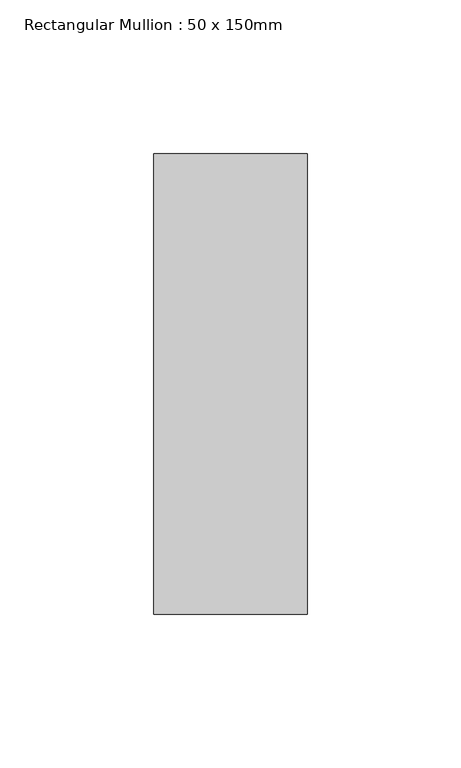
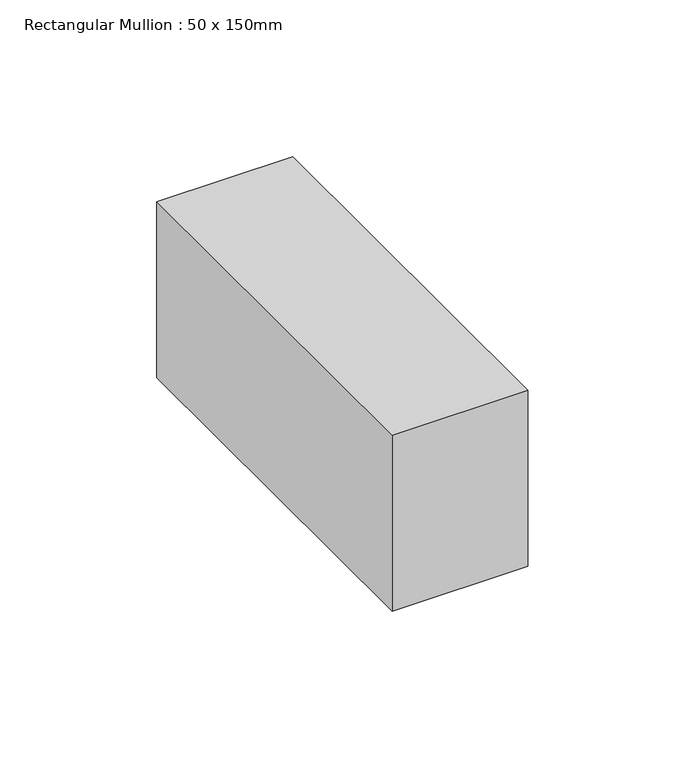
"""IFC4 building model written with IfcOpenShell, lengths in millimetres: member geometry, Rectangular Mullion : 50 x 150mm."""

from ifc_helpers import new_model, si_unit, frame, origin, place, context, project, spatial, polyline, outline, extrude, source, transform, mapped, element, save


def rectangular_mullion_50_x_150mm_e4b12c2e(model_context):
    return source(origin(), model_context, "Body", "SweptSolid", [
        extrude(outline(polyline([(0.0, 75.0), (0.0, -75.0), (-50.0, -75.0), (-50.0, 75.0), (0.0, 75.0)])), frame((0.0, 0.0, -68.4152885), z_axis=(0.0, 0.0, 1.0), x_axis=(1.0, 0.0, 0.0)), (0.0, 0.0, 1.0), 68.4152885),
    ])


if __name__ == "__main__":
    model = new_model("IFC4")
    model_context = context("Model", 3, world=origin())
    ifc_project = project(units=[si_unit("LENGTHUNIT", "METRE", prefix="MILLI")], contexts=[model_context])
    site = spatial("IfcSite", under=ifc_project)
    building = spatial("IfcBuilding", under=site)
    placement = place(None, origin())
    rectangular_mullion_50_x_150mm_shape = rectangular_mullion_50_x_150mm_e4b12c2e(model_context)
    element("IfcMember", 1, ObjectType="Rectangular Mullion : 50 x 150mm", at=placement, inside=building, context=model_context, shape_type="MappedRepresentation", body=[
        mapped(rectangular_mullion_50_x_150mm_shape, transform((0.0, 0.0, 0.0), x_axis=(1.0, 0.0, 0.0), y_axis=(0.0, 1.0, 0.0), z_axis=(0.0, 0.0, 1.0))),
    ])
    save(model, "model.ifc")

# Revit data of these elements
# Type "Rectangular Mullion : 50 x 150mm"
#   built-in parameter 1007304 = 0.492126 (stored number, unit not read)
#   built-in parameter 1007301 = 0.082021 (stored number, unit not read)
#   built-in parameter 1007300 = 0.082021 (stored number, unit not read)
# Element 1 (IfcMember, "Rectangular Mullion : 50 x 150mm")
#   Materials on its faces: "Aluminium"
# Materials
#   "Aluminium": class "Metal", colour RGB 247 247 247, transparency 0, Description = "Aluminium 6061", Cost = 0
